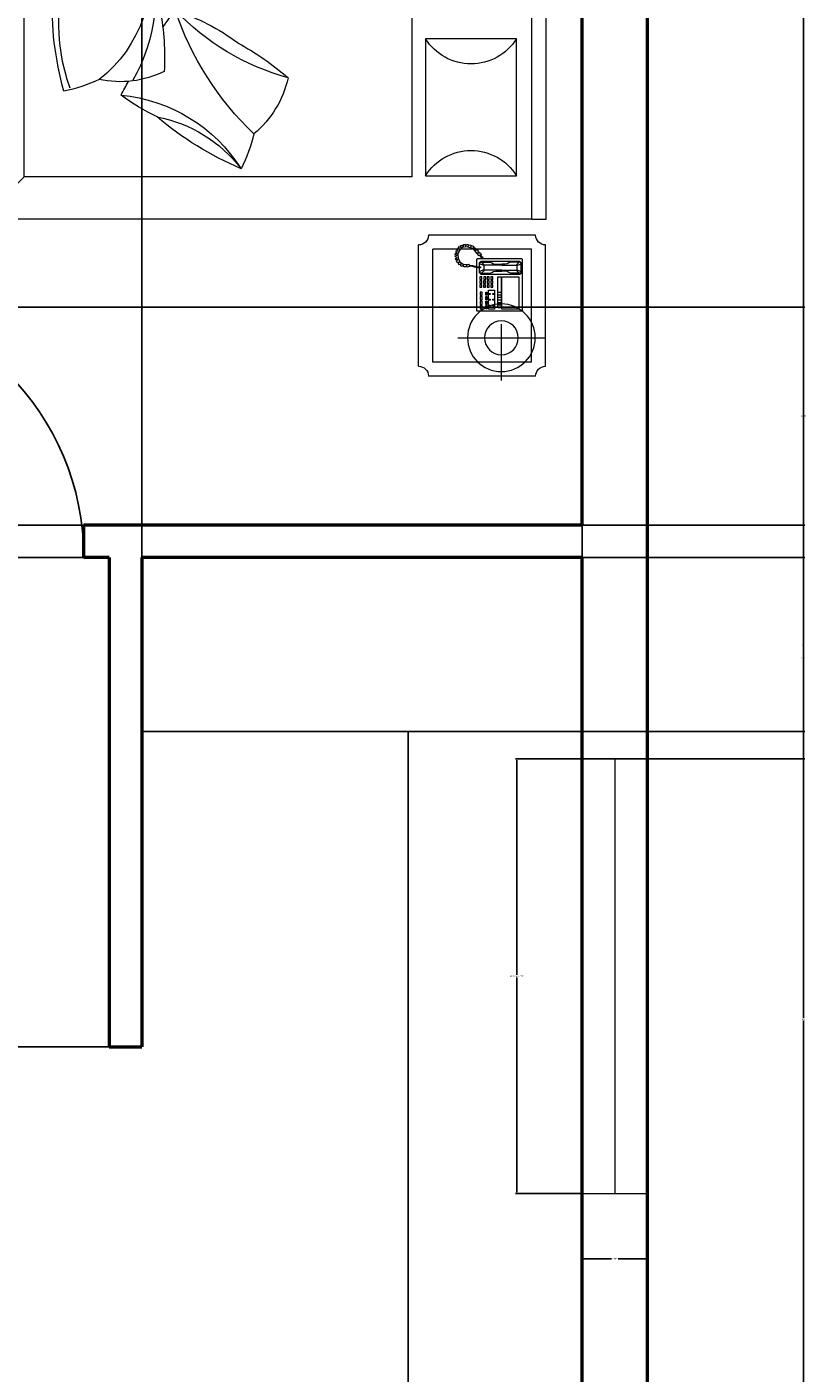
# Model space of a CAD drawing. Units: inches. Extents: x -108 to 1456, y -102 to 617.
# Tile 6 of 8: x 453 to 560, y 337 to 523. Entities that reach past the tile are written whole.
import ezdxf

# ---------------------------------------------------------------- set-up
doc = ezdxf.new("R2010")
doc.units = ezdxf.units.IN
for name, color, linetype, lineweight in [('A-ANNO-DIMS', 2, 'Continuous', 18), ('A-DOOR', 3, 'Continuous', 25), ('A-FLOR-CASE', 32, 'Continuous', 25), ('A-FURN', 8, 'Continuous', 18), ('A-GLAZ', 4, 'Continuous', 18), ('A-WALL', 7, 'Continuous', 50)]:
    doc.layers.add(name, color=color, linetype=linetype, lineweight=lineweight)
doc.styles.get("Standard").update_dxf_attribs({"font": 'arial.ttf'})
doc.dimstyles.get("Standard").update_dxf_attribs({"dimtxt": 0.18, "dimasz": 0.18, "dimexe": 0.18, "dimexo": 0.0625, "dimgap": 0.09, "dimtad": 0, "dimtih": 1, "dimtoh": 1, "dimdec": 4, "dimzin": 0, "dimdsep": 46, "dimtxsty": 'Standard', "dimcen": 0.09, "dimadec": 0, "dimazin": 0, "dimtfac": 1, "dimtdec": 4, "dimtofl": 0, "dimtmove": 0, "dimatfit": 3, "dimfxl": 1, "dimtolj": 1, "dimtzin": 0, "dimarcsym": 0})

# ---------------------------------------------------------------- blocks, each defined once
blk = doc.blocks.new('A$C50B66110')
for p, q in [((0.0153, 1.9631), (0.0153, 1.5831)), ((0.0503, 1.9981), (0.4803, 1.9981)), ((0.1513, 1.6871), (0.1513, 1.9967)), ((0.5153, 1.9631), (0.5153, 1.5831)), ((0.5716, 1.9488), (0.5716, 2)), ((0.5716, 2), (2.0719, 2)), ((2.0719, 1.9488), (2.0719, 2)), ((2.1051, 1.9643), (2.1051, 1.5843)), ((2.5701, 1.9993), (2.1401, 1.9993)), ((2.6051, 1.9643), (2.6051, 1.5843)), ((0.0653, 1.9481), (0.0653, 1.5981)), ((0.0653, 1.9481), (0.4653, 1.9481)), ((0.4653, 1.9481), (0.4653, 1.5981)), ((2.0719, 1.9488), (0.5716, 1.9488)), ((0.5716, 1.9488), (0.5716, 0)), ((2.0719, 0), (2.0719, 1.9488)), ((2.1551, 1.9493), (2.1551, 1.5993)), ((2.5551, 1.9493), (2.1551, 1.9493)), ((2.3505, 1.62), (2.3505, 1.9295)), ((2.5551, 1.9493), (2.5551, 1.5993)), ((0.7257, 1.5725), (0.7257, 1.8954)), ((0.7257, 1.8954), (1.2113, 1.8954)), ((1.2113, 1.8954), (1.2113, 1.5725)), ((1.4007, 1.5725), (1.4007, 1.8954)), ((1.4007, 1.8954), (1.8863, 1.8954)), ((1.8863, 1.8954), (1.8863, 1.5725)), ((0, 1.8416), (0.2001, 1.8416)), ((2.5018, 1.7744), (2.2017, 1.7744)), ((0.0653, 1.5981), (0.4653, 1.5981)), ((2.5551, 1.5993), (2.1551, 1.5993)), ((0.0503, 1.5481), (0.4803, 1.5481)), ((1.2113, 1.5725), (0.7257, 1.5725)), ((1.8863, 1.5725), (1.4007, 1.5725)), ((2.5701, 1.5493), (2.1401, 1.5493)), ((1.5665, 1.5254), (1.5665, 1.0802)), ((1.5665, 1.5254), (1.9219, 1.0802)), ((1.9219, 1.0802), (1.5665, 1.0802)), ((0.5716, 0), (0.7216, 0.15)), ((2.0719, 0), (1.9219, 0.15)), ((0.5716, 0), (2.0719, 0))]:
    blk.add_line(p, q)
at = {"linetype": 'ByBlock'}
for p, q in [((0.2481, 1.9162), (0.2458, 1.9139)), ((0.2458, 1.9139), (0.2458, 1.7562)), ((0.2481, 1.9162), (0.4287, 1.9162)), ((0.3772, 1.9071), (0.3818, 1.9128)), ((0.3818, 1.9094), (0.3807, 1.9048)), ((0.3818, 1.9128), (0.4161, 1.9128)), ((0.3864, 1.9116), (0.3818, 1.9094)), ((0.3921, 1.8968), (0.3864, 1.9116)), ((0.3864, 1.9116), (0.4138, 1.9116)), ((0.4081, 1.8968), (0.4138, 1.9116)), ((0.4138, 1.9116), (0.4184, 1.9094)), ((0.4161, 1.9128), (0.4218, 1.9071)), ((0.4184, 1.9094), (0.4195, 1.9048)), ((0.4287, 1.9162), (0.4309, 1.9139)), ((0.4309, 1.9139), (0.4309, 1.7562)), ((0.2526, 1.9036), (0.2526, 1.8431)), ((0.3669, 1.9036), (0.2526, 1.9036)), ((0.3669, 1.8431), (0.3669, 1.9036)), ((0.3772, 1.7688), (0.3772, 1.9071)), ((0.3807, 1.9048), (0.3807, 1.8739)), ((0.3807, 1.9048), (0.3909, 1.8945)), ((0.3807, 1.8739), (0.3829, 1.8682)), ((0.3829, 1.8682), (0.3864, 1.8625)), ((0.3864, 1.8625), (0.3875, 1.8545)), ((0.3909, 1.8945), (0.3921, 1.8968)), ((0.3909, 1.8431), (0.3909, 1.8945)), ((0.4081, 1.8968), (0.3921, 1.8968)), ((0.4092, 1.8945), (0.4081, 1.8968)), ((0.4195, 1.9048), (0.4092, 1.8945)), ((0.4092, 1.8431), (0.4092, 1.8945)), ((0.4138, 1.8625), (0.4127, 1.8545)), ((0.4172, 1.8682), (0.4138, 1.8625)), ((0.4195, 1.8739), (0.4172, 1.8682)), ((0.4195, 1.9048), (0.4195, 1.8739)), ((0.4218, 1.9071), (0.4218, 1.7699)), ((0.2526, 1.8431), (0.3669, 1.8431)), ((0.3201, 1.8168), (0.2526, 1.8168)), ((0.2526, 1.8168), (0.2526, 1.7962)), ((0.2572, 1.8408), (0.2572, 1.8294)), ((0.3669, 1.8408), (0.2572, 1.8408)), ((0.2572, 1.8294), (0.3669, 1.8294)), ((0.2675, 1.8145), (0.2641, 1.8145)), ((0.2641, 1.8145), (0.2641, 1.8111)), ((0.2664, 1.8408), (0.2664, 1.8294)), ((0.2675, 1.8111), (0.2675, 1.8145)), ((0.2755, 1.8408), (0.2755, 1.8294)), ((0.2846, 1.8408), (0.2846, 1.8294)), ((0.2846, 1.8145), (0.2846, 1.8111)), ((0.2881, 1.8145), (0.2846, 1.8145)), ((0.2881, 1.8111), (0.2881, 1.8145)), ((0.2938, 1.8408), (0.2938, 1.8294)), ((0.3029, 1.8408), (0.3029, 1.8294)), ((0.3052, 1.8145), (0.3052, 1.8111)), ((0.3086, 1.8145), (0.3052, 1.8145)), ((0.3086, 1.8111), (0.3086, 1.8145)), ((0.3121, 1.8408), (0.3121, 1.8294)), ((0.3201, 1.7962), (0.3201, 1.8168)), ((0.3669, 1.8294), (0.3669, 1.8408)), ((0.3829, 1.8076), (0.3864, 1.8134)), ((0.3864, 1.8134), (0.3875, 1.8214)), ((0.3875, 1.8545), (0.3875, 1.8431)), ((0.3875, 1.8214), (0.3875, 1.8431)), ((0.3909, 1.8431), (0.3909, 1.7813)), ((0.4092, 1.8431), (0.4092, 1.7813)), ((0.4127, 1.8545), (0.4127, 1.8431)), ((0.4127, 1.8214), (0.4127, 1.8431)), ((0.4138, 1.8134), (0.4127, 1.8214)), ((0.4172, 1.8076), (0.4138, 1.8134)), ((0.2526, 1.7962), (0.3201, 1.7962)), ((0.2652, 1.7905), (0.2538, 1.7905)), ((0.2538, 1.7905), (0.2538, 1.7859)), ((0.2538, 1.7859), (0.2652, 1.7859)), ((0.2538, 1.7665), (0.2538, 1.7733)), ((0.2538, 1.7733), (0.2652, 1.7733)), ((0.2652, 1.7665), (0.2538, 1.7665)), ((0.2641, 1.8111), (0.2675, 1.8111)), ((0.2641, 1.8019), (0.2641, 1.7985)), ((0.2675, 1.8019), (0.2641, 1.8019)), ((0.2641, 1.7985), (0.2675, 1.7985)), ((0.2652, 1.7859), (0.2652, 1.7905)), ((0.2652, 1.7733), (0.2652, 1.7665)), ((0.2675, 1.7985), (0.2675, 1.8019)), ((0.2812, 1.7905), (0.2698, 1.7905)), ((0.2698, 1.7905), (0.2698, 1.7859)), ((0.2698, 1.7859), (0.2812, 1.7859)), ((0.2698, 1.7665), (0.2698, 1.7733)), ((0.2698, 1.7733), (0.2812, 1.7733)), ((0.2812, 1.7665), (0.2698, 1.7665)), ((0.2812, 1.7859), (0.2812, 1.7905)), ((0.2812, 1.7733), (0.2812, 1.7665)), ((0.2846, 1.8111), (0.2881, 1.8111)), ((0.2846, 1.8019), (0.2846, 1.7985)), ((0.2881, 1.8019), (0.2846, 1.8019)), ((0.2846, 1.7985), (0.2881, 1.7985)), ((0.2972, 1.7905), (0.2858, 1.7905)), ((0.2858, 1.7905), (0.2858, 1.7859)), ((0.2858, 1.7859), (0.2972, 1.7859)), ((0.2858, 1.7665), (0.2858, 1.7733)), ((0.2858, 1.7733), (0.2972, 1.7733)), ((0.2972, 1.7665), (0.2858, 1.7665)), ((0.2881, 1.7985), (0.2881, 1.8019)), ((0.2972, 1.7859), (0.2972, 1.7905)), ((0.2972, 1.7733), (0.2972, 1.7665)), ((0.3018, 1.7905), (0.3018, 1.7859)), ((0.3132, 1.7905), (0.3018, 1.7905)), ((0.3018, 1.7859), (0.3132, 1.7859)), ((0.3018, 1.7733), (0.3132, 1.7733)), ((0.3018, 1.7665), (0.3018, 1.7733)), ((0.3132, 1.7665), (0.3018, 1.7665)), ((0.3052, 1.8111), (0.3086, 1.8111)), ((0.3052, 1.8019), (0.3052, 1.7985)), ((0.3086, 1.8019), (0.3052, 1.8019)), ((0.3052, 1.7985), (0.3086, 1.7985)), ((0.3086, 1.7985), (0.3086, 1.8019)), ((0.3132, 1.7859), (0.3132, 1.7905)), ((0.3132, 1.7733), (0.3132, 1.7665)), ((0.3304, 1.8111), (0.3395, 1.8111)), ((0.3304, 1.8042), (0.3304, 1.8111)), ((0.3395, 1.8042), (0.3304, 1.8042)), ((0.3304, 1.7985), (0.3395, 1.7985)), ((0.3304, 1.7916), (0.3304, 1.7985)), ((0.3395, 1.7916), (0.3304, 1.7916)), ((0.3304, 1.7779), (0.3304, 1.7848)), ((0.3304, 1.7848), (0.3395, 1.7848)), ((0.3395, 1.7779), (0.3304, 1.7779)), ((0.3304, 1.7722), (0.3395, 1.7722)), ((0.3304, 1.7653), (0.3304, 1.7722)), ((0.3395, 1.8111), (0.3395, 1.8042)), ((0.3395, 1.7985), (0.3395, 1.7916)), ((0.3395, 1.7848), (0.3395, 1.7779)), ((0.3395, 1.7722), (0.3395, 1.7653)), ((0.3441, 1.8042), (0.3441, 1.8111)), ((0.3441, 1.8111), (0.3532, 1.8111)), ((0.3532, 1.8042), (0.3441, 1.8042)), ((0.3441, 1.7985), (0.3532, 1.7985)), ((0.3441, 1.7916), (0.3441, 1.7985)), ((0.3532, 1.7916), (0.3441, 1.7916)), ((0.3441, 1.7779), (0.3441, 1.7848)), ((0.3441, 1.7848), (0.3532, 1.7848)), ((0.3532, 1.7779), (0.3441, 1.7779)), ((0.3441, 1.7722), (0.3532, 1.7722)), ((0.3441, 1.7653), (0.3441, 1.7722)), ((0.3532, 1.8111), (0.3532, 1.8042)), ((0.3532, 1.7985), (0.3532, 1.7916)), ((0.3532, 1.7848), (0.3532, 1.7779)), ((0.3532, 1.7722), (0.3532, 1.7653)), ((0.3578, 1.8111), (0.3669, 1.8111)), ((0.3578, 1.8042), (0.3578, 1.8111)), ((0.3669, 1.8042), (0.3578, 1.8042)), ((0.3578, 1.7985), (0.3669, 1.7985)), ((0.3578, 1.7916), (0.3578, 1.7985)), ((0.3669, 1.7916), (0.3578, 1.7916)), ((0.3578, 1.7791), (0.3578, 1.7859)), ((0.3578, 1.7859), (0.3669, 1.7859)), ((0.3669, 1.7791), (0.3578, 1.7791)), ((0.3578, 1.7653), (0.3578, 1.7722)), ((0.3578, 1.7722), (0.3669, 1.7722)), ((0.3669, 1.8111), (0.3669, 1.8042)), ((0.3669, 1.7985), (0.3669, 1.7916)), ((0.3669, 1.7859), (0.3669, 1.7791)), ((0.3669, 1.7722), (0.3669, 1.7653)), ((0.3829, 1.7631), (0.3772, 1.7688)), ((0.3807, 1.8019), (0.3829, 1.8076)), ((0.3807, 1.7711), (0.3807, 1.8019)), ((0.3807, 1.7711), (0.3909, 1.7813)), ((0.3818, 1.7665), (0.3807, 1.7711)), ((0.3864, 1.7642), (0.3818, 1.7665)), ((0.3921, 1.7791), (0.3864, 1.7642)), ((0.3909, 1.7813), (0.3921, 1.7791)), ((0.4081, 1.7791), (0.3921, 1.7791)), ((0.4024, 1.7676), (0.3989, 1.7676)), ((0.3989, 1.7676), (0.3991, 1.7578)), ((0.403, 1.7585), (0.4024, 1.7676)), ((0.4092, 1.7813), (0.4081, 1.7791)), ((0.4081, 1.7791), (0.4138, 1.7642)), ((0.4195, 1.7711), (0.4092, 1.7813)), ((0.4138, 1.7642), (0.4184, 1.7665)), ((0.4218, 1.7699), (0.4161, 1.7631)), ((0.4195, 1.8019), (0.4172, 1.8076)), ((0.4184, 1.7665), (0.4195, 1.7711)), ((0.4195, 1.7711), (0.4195, 1.8019)), ((0.4378, 1.7742), (0.4309, 1.7768)), ((0.4309, 1.7722), (0.436, 1.7708)), ((0.436, 1.7708), (0.4406, 1.7672)), ((0.441, 1.771), (0.4378, 1.7742)), ((0.4406, 1.7672), (0.4418, 1.7656)), ((0.4434, 1.7688), (0.441, 1.771)), ((0.4443, 1.7658), (0.4418, 1.7633)), ((0.4418, 1.7656), (0.4443, 1.7658)), ((0.4477, 1.7704), (0.4434, 1.7688)), ((0.4497, 1.7684), (0.4477, 1.7704)), ((0.4481, 1.765), (0.4497, 1.7684)), ((0.4509, 1.7672), (0.4481, 1.765)), ((0.4539, 1.764), (0.4509, 1.7672)), ((0.2458, 1.7562), (0.2481, 1.7539)), ((0.4, 1.7539), (0.2481, 1.7539)), ((0.3395, 1.7653), (0.3304, 1.7653)), ((0.3532, 1.7653), (0.3441, 1.7653)), ((0.3669, 1.7653), (0.3578, 1.7653)), ((0.399, 1.7631), (0.3829, 1.7631)), ((0.3864, 1.7642), (0.399, 1.7642)), ((0.3991, 1.7578), (0.4019, 1.7462)), ((0.4019, 1.7462), (0.4047, 1.7353)), ((0.4026, 1.7254), (0.4021, 1.7198)), ((0.4021, 1.7198), (0.4088, 1.7187)), ((0.4088, 1.7187), (0.4023, 1.7147)), ((0.4026, 1.7642), (0.4138, 1.7642)), ((0.4051, 1.7279), (0.4026, 1.7254)), ((0.4161, 1.7631), (0.4027, 1.7631)), ((0.4047, 1.7511), (0.403, 1.7585)), ((0.4287, 1.7539), (0.404, 1.7539)), ((0.4047, 1.7353), (0.4044, 1.7293)), ((0.4044, 1.7293), (0.4051, 1.7279)), ((0.4074, 1.7402), (0.4047, 1.7511)), ((0.4081, 1.7346), (0.4074, 1.7402)), ((0.4079, 1.7286), (0.4081, 1.7346)), ((0.4121, 1.7256), (0.4079, 1.7286)), ((0.4111, 1.7203), (0.4121, 1.7256)), ((0.4123, 1.7057), (0.4111, 1.7203)), ((0.4309, 1.7562), (0.4287, 1.7539)), ((0.4418, 1.7633), (0.4511, 1.7551)), ((0.4511, 1.7551), (0.4662, 1.7422)), ((0.4515, 1.7573), (0.4539, 1.764)), ((0.4577, 1.7605), (0.4515, 1.7573)), ((0.463, 1.7555), (0.4577, 1.7605)), ((0.4618, 1.7482), (0.463, 1.7555)), ((0.467, 1.7515), (0.4618, 1.7482)), ((0.4664, 1.7418), (0.4741, 1.72)), ((0.4714, 1.7468), (0.467, 1.7515)), ((0.4696, 1.7418), (0.4714, 1.7468)), ((0.4766, 1.7425), (0.4697, 1.7418)), ((0.4741, 1.72), (0.4708, 1.7027)), ((0.472, 1.733), (0.4787, 1.7356)), ((0.4794, 1.7332), (0.472, 1.733)), ((0.4761, 1.7233), (0.481, 1.7279)), ((0.4824, 1.7233), (0.4761, 1.7233)), ((0.4787, 1.7356), (0.4766, 1.7425)), ((0.481, 1.7279), (0.4794, 1.7332)), ((0.4835, 1.7175), (0.4824, 1.7233)), ((0.4023, 1.7147), (0.4028, 1.7085)), ((0.4028, 1.7085), (0.4102, 1.7078)), ((0.4102, 1.7078), (0.4037, 1.7027)), ((0.4037, 1.7027), (0.4067, 1.6974)), ((0.4067, 1.6974), (0.4137, 1.6988)), ((0.4137, 1.6988), (0.4104, 1.6923)), ((0.4104, 1.6923), (0.4139, 1.6881)), ((0.4211, 1.6946), (0.4123, 1.7057)), ((0.4139, 1.6881), (0.4192, 1.692)), ((0.4192, 1.692), (0.4183, 1.6858)), ((0.4183, 1.6858), (0.4227, 1.683)), ((0.4333, 1.6881), (0.4211, 1.6946)), ((0.4227, 1.683), (0.4283, 1.6876)), ((0.4283, 1.6876), (0.4276, 1.68)), ((0.4276, 1.68), (0.4324, 1.6786)), ((0.4324, 1.6786), (0.4354, 1.6849)), ((0.4472, 1.6869), (0.4333, 1.6881)), ((0.4354, 1.6849), (0.4382, 1.6786)), ((0.4382, 1.6786), (0.4421, 1.6782)), ((0.4421, 1.6782), (0.4437, 1.6849)), ((0.4437, 1.6849), (0.4463, 1.6775)), ((0.4463, 1.6775), (0.4507, 1.6786)), ((0.4606, 1.6927), (0.4472, 1.6869)), ((0.4507, 1.6786), (0.4509, 1.6849)), ((0.4509, 1.6849), (0.4562, 1.6802)), ((0.4562, 1.6802), (0.4599, 1.6821)), ((0.4592, 1.689), (0.4641, 1.683)), ((0.4599, 1.6821), (0.4592, 1.689)), ((0.4708, 1.7027), (0.4606, 1.6927)), ((0.4641, 1.683), (0.4678, 1.6863)), ((0.465, 1.6925), (0.4715, 1.6897)), ((0.4678, 1.6863), (0.465, 1.6925)), ((0.4745, 1.6925), (0.4713, 1.6988)), ((0.4713, 1.6988), (0.478, 1.6967)), ((0.4715, 1.6897), (0.4745, 1.6925)), ((0.4743, 1.7075), (0.4815, 1.7073)), ((0.4798, 1.7013), (0.4743, 1.7075)), ((0.4764, 1.7154), (0.4835, 1.7175)), ((0.4824, 1.7119), (0.4764, 1.7154)), ((0.478, 1.6967), (0.4798, 1.7013)), ((0.4815, 1.7073), (0.4824, 1.7119)), ((0.7216, 1.5254), (1.9219, 1.5254)), ((0.7216, 1.5254), (0.7216, 0.15)), ((1.9219, 0.15), (1.9219, 1.5254)), ((0.7216, 0.15), (1.9219, 0.15))]:
    blk.add_line(p, q, dxfattribs=at)
for centre, radius in [((0.1513, 1.8416), 0.12), ((0.1513, 1.8416), 0.06), ((2.3505, 1.7744), 0.12), ((2.3505, 1.7744), 0.06)]:
    blk.add_circle(centre, radius)
for centre, radius, start, end in [((0.0153, 1.9981), 0.035, 270, 0), ((0.5153, 1.9981), 0.035, 180, 270), ((2.1051, 1.9993), 0.035, 270, 0), ((2.6051, 1.9993), 0.035, 180, 270), ((0.6244, 1.734), 0.1906, 302.1202, 57.8798), ((1.3126, 1.734), 0.1906, 122.1202, 237.8798), ((1.2994, 1.734), 0.1906, 302.1202, 57.8798), ((1.9876, 1.734), 0.1906, 122.1202, 237.8798), ((0.0153, 1.5481), 0.035, 0, 90), ((0.5153, 1.5481), 0.035, 90, 180), ((2.1051, 1.5493), 0.035, 0, 90), ((2.6051, 1.5493), 0.035, 90, 180), ((1.1502, 0.7366), 0.3575, 102.4782, 140.4625), ((0.328, 0.4368), 0.9879, 28.4971, 41.0566), ((1.9117, 1.3157), 0.8697, 195.336, 226.4193), ((0.9996, 0.4307), 0.548, 103.2034, 117.0362), ((1.656, 1.7093), 1.0798, 223.6306, 251.4288), ((0.4482, 0.4408), 0.5655, 5.3391, 57.6895), ((1.8226, 1.3753), 1.1652, 203.0642, 220.3209), ((0.4548, 0.5307), 0.4879, 10.6986, 52.6864), ((0.5648, 0.4378), 0.7874, 18.3527, 36.6851), ((-0.0179, 2.4352), 2.1977, 305.2966, 307.2418), ((1.5981, 0.9345), 0.734, 205.259, 216.9351), ((1.4166, 0.4903), 0.3575, 154.0418, 192.0262), ((1.1403, -0.3401), 0.9879, 80.0607, 92.6202), ((1.2867, -0.154), 0.7874, 69.9163, 88.2487), ((1.3672, 0.0075), 0.6085, 71.81, 120.1351), ((1.4431, 0.1219), 0.4774, 76.1849, 142.0017), ((-0.6401, 0.6314), 2.1977, 349.4884, 358.8054), ((-0.0179, 2.4352), 2.1977, 297.9248, 299.3793), ((1.5626, 0.1822), 0.548, 154.767, 168.5998), ((1.3343, 1.4141), 1.1652, 254.6278, 271.8845), ((1.2678, 0.9611), 0.6885, 250.2936, 293.6414), ((1.5399, 0.9642), 0.734, 256.8226, 268.4988)]:
    blk.add_arc(centre, radius, start, end)
blk = doc.blocks.new('WIN-60-WALL-9')
for p, q in [((0, 0), (0, 9)), ((60, 0), (60, 9)), ((0, 4.5), (60, 4.5))]:
    blk.add_line(p, q)
blk = doc.blocks.new('*D16')
at = {"layer": 'A-ANNO-DIMS', "color": 0, "lineweight": -2, "transparency": 16777216}
for p, q in [((529.28, 421.77), (520.16, 421.77)), ((520.34, 421.59), (520.34, 391.96)), ((520.34, 361.95), (520.34, 391.59)), ((529.28, 361.77), (520.16, 361.77))]:
    blk.add_line(p, q, dxfattribs=at)
at = {"layer": 'A-ANNO-DIMS', "color": 0, "transparency": 16777216}
for points in [[(520.31, 421.59), (520.37, 421.59), (520.34, 421.77)], [(520.31, 361.95), (520.37, 361.95), (520.34, 361.77)]]:
    blk.add_solid(points, dxfattribs=at)
at = {"layer": 'Defpoints', "color": 0, "transparency": 16777216}
for p in [(529.34, 421.77), (520.34, 361.77), (529.34, 361.77)]:
    blk.add_point(p, dxfattribs=at)
at = {"layer": 'A-ANNO-DIMS', "color": 0, "transparency": 16777216, "insert": (520.34, 391.77), "char_height": 0.18, "attachment_point": 5}
blk.add_mtext('\\A1;WINDOW 60 TYP.', dxfattribs=at)
blk = doc.blocks.new('*D17')
at = {"layer": 'A-ANNO-DIMS', "color": 0, "lineweight": -2, "transparency": 16777216}
for p, q in [((529.34, 361.71), (529.34, 352.59)), ((538.34, 361.71), (538.34, 352.59)), ((529.52, 352.77), (533.39, 352.77)), ((538.16, 352.77), (534.3, 352.77))]:
    blk.add_line(p, q, dxfattribs=at)
at = {"layer": 'A-ANNO-DIMS', "color": 0, "transparency": 16777216}
for points in [[(529.52, 352.8), (529.52, 352.74), (529.34, 352.77)], [(538.16, 352.8), (538.16, 352.74), (538.34, 352.77)]]:
    blk.add_solid(points, dxfattribs=at)
at = {"layer": 'Defpoints', "color": 0, "transparency": 16777216}
for p in [(529.34, 361.77), (538.34, 361.77), (538.34, 352.77)]:
    blk.add_point(p, dxfattribs=at)
at = {"layer": 'A-ANNO-DIMS', "color": 0, "transparency": 16777216, "insert": (533.84, 352.77), "char_height": 0.18, "attachment_point": 5}
blk.add_mtext('\\A1;9 TYP.', dxfattribs=at)
blk = doc.blocks.new('*D35')
at = {"layer": 'A-ANNO-DIMS', "color": 0, "lineweight": -2, "transparency": 16777216}
for p, q in [((538.41, 595.77), (560.05, 595.77)), ((559.87, 595.59), (559.87, 385.96)), ((559.87, 175.95), (559.87, 385.59)), ((538.41, 175.77), (560.05, 175.77))]:
    blk.add_line(p, q, dxfattribs=at)
at = {"layer": 'A-ANNO-DIMS', "color": 0, "transparency": 16777216}
for points in [[(559.84, 595.59), (559.9, 595.59), (559.87, 595.77)], [(559.84, 175.95), (559.9, 175.95), (559.87, 175.77)]]:
    blk.add_solid(points, dxfattribs=at)
at = {"layer": 'Defpoints', "color": 0, "transparency": 16777216}
for p in [(538.34, 595.77), (559.87, 595.77), (538.34, 175.77)]:
    blk.add_point(p, dxfattribs=at)
at = {"layer": 'A-ANNO-DIMS', "color": 0, "transparency": 16777216, "insert": (559.87, 385.77), "char_height": 0.18, "attachment_point": 5}
blk.add_mtext('\\A1;420', dxfattribs=at)
blk = doc.blocks.new('*D52')
at = {"layer": 'A-ANNO-DIMS', "color": 0, "lineweight": -2, "transparency": 16777216}
for p, q in [((415.48, 484.07), (560.05, 484.07)), ((559.87, 483.89), (559.87, 469.23)), ((559.87, 454.2), (559.87, 468.86)), ((416.16, 454.02), (560.05, 454.02))]:
    blk.add_line(p, q, dxfattribs=at)
at = {"layer": 'A-ANNO-DIMS', "color": 0, "transparency": 16777216}
for points in [[(559.84, 483.89), (559.9, 483.89), (559.87, 484.07)], [(559.84, 454.2), (559.9, 454.2), (559.87, 454.02)]]:
    blk.add_solid(points, dxfattribs=at)
at = {"layer": 'Defpoints', "color": 0, "transparency": 16777216}
for p in [(415.41, 484.07), (416.09, 454.02), (559.87, 454.02)]:
    blk.add_point(p, dxfattribs=at)
at = {"layer": 'A-ANNO-DIMS', "color": 0, "transparency": 16777216, "insert": (559.87, 469.05), "char_height": 0.18, "attachment_point": 5}
blk.add_mtext('\\A1;30.044', dxfattribs=at)
blk = doc.blocks.new('*D54')
at = {"layer": 'A-ANNO-DIMS', "color": 0, "lineweight": -2, "transparency": 16777216}
for p, q in [((529.41, 449.52), (560.05, 449.52)), ((559.87, 449.34), (559.87, 435.83)), ((559.87, 421.95), (559.87, 435.47)), ((529.41, 421.77), (560.05, 421.77))]:
    blk.add_line(p, q, dxfattribs=at)
at = {"layer": 'A-ANNO-DIMS', "color": 0, "transparency": 16777216}
for points in [[(559.84, 449.34), (559.9, 449.34), (559.87, 449.52)], [(559.84, 421.95), (559.9, 421.95), (559.87, 421.77)]]:
    blk.add_solid(points, dxfattribs=at)
at = {"layer": 'Defpoints', "color": 0, "transparency": 16777216}
for p in [(529.34, 449.52), (529.34, 421.77), (559.87, 421.77)]:
    blk.add_point(p, dxfattribs=at)
at = {"layer": 'A-ANNO-DIMS', "color": 0, "transparency": 16777216, "insert": (559.87, 435.65), "char_height": 0.18, "attachment_point": 5}
blk.add_mtext('\\A1;27.75', dxfattribs=at)
blk = doc.blocks.new('*D57')
at = {"layer": 'A-ANNO-DIMS', "color": 0, "lineweight": -2, "transparency": 16777216}
for p, q in [((468.59, 449.59), (468.59, 617.48)), ((468.77, 617.3), (498.57, 617.3)), ((529.16, 617.3), (499.36, 617.3)), ((529.34, 449.59), (529.34, 617.48))]:
    blk.add_line(p, q, dxfattribs=at)
at = {"layer": 'A-ANNO-DIMS', "color": 0, "transparency": 16777216}
for points in [[(468.77, 617.33), (468.77, 617.27), (468.59, 617.3)], [(529.16, 617.33), (529.16, 617.27), (529.34, 617.3)]]:
    blk.add_solid(points, dxfattribs=at)
at = {"layer": 'Defpoints', "color": 0, "transparency": 16777216}
for p in [(529.34, 617.3), (468.59, 449.52), (529.34, 449.52)]:
    blk.add_point(p, dxfattribs=at)
at = {"layer": 'A-ANNO-DIMS', "color": 0, "transparency": 16777216, "insert": (498.97, 617.3), "char_height": 0.18, "attachment_point": 5}
blk.add_mtext('\\A1;60.75', dxfattribs=at)
blk = doc.blocks.new('*D58')
at = {"layer": 'A-ANNO-DIMS', "color": 0, "lineweight": -2, "transparency": 16777216}
for p, q in [((464.03, 449.52), (204.64, 449.52)), ((204.82, 449.34), (204.82, 415.95)), ((204.82, 382.19), (204.82, 415.58)), ((464.03, 382.01), (204.64, 382.01))]:
    blk.add_line(p, q, dxfattribs=at)
at = {"layer": 'A-ANNO-DIMS', "color": 0, "transparency": 16777216}
for points in [[(204.79, 449.34), (204.85, 449.34), (204.82, 449.52)], [(204.79, 382.19), (204.85, 382.19), (204.82, 382.01)]]:
    blk.add_solid(points, dxfattribs=at)
at = {"layer": 'Defpoints', "color": 0, "transparency": 16777216}
for p in [(464.09, 449.52), (204.82, 382.01), (464.09, 382.01)]:
    blk.add_point(p, dxfattribs=at)
at = {"layer": 'A-ANNO-DIMS', "color": 0, "transparency": 16777216, "insert": (204.82, 415.77), "char_height": 0.18, "attachment_point": 5}
blk.add_mtext('\\A1;67.52', dxfattribs=at)
blk = doc.blocks.new('*D60')
at = {"layer": 'A-ANNO-DIMS', "color": 0, "lineweight": -2, "transparency": 16777216}
for p, q in [((468.66, 449.52), (560.05, 449.52)), ((559.87, 449.34), (559.87, 437.7)), ((559.87, 425.7), (559.87, 437.34)), ((468.66, 425.52), (560.05, 425.52))]:
    blk.add_line(p, q, dxfattribs=at)
at = {"layer": 'A-ANNO-DIMS', "color": 0, "transparency": 16777216}
for points in [[(559.84, 449.34), (559.9, 449.34), (559.87, 449.52)], [(559.84, 425.7), (559.9, 425.7), (559.87, 425.52)]]:
    blk.add_solid(points, dxfattribs=at)
at = {"layer": 'Defpoints', "color": 0, "transparency": 16777216}
for p in [(468.59, 449.52), (559.87, 449.52), (468.59, 425.52)]:
    blk.add_point(p, dxfattribs=at)
at = {"layer": 'A-ANNO-DIMS', "color": 0, "transparency": 16777216, "insert": (559.87, 437.52), "char_height": 0.18, "attachment_point": 5}
blk.add_mtext('\\A1;24', dxfattribs=at)

msp = doc.modelspace()

# ---------------------------------------------------------------- linework, layer by layer
at = {"layer": 'A-DOOR'}
msp.add_arc((424.5943, 449.5243), 36, 0, 90, dxfattribs=at)
at = {"layer": 'A-FLOR-CASE'}
for p, q in [((468.5943, 449.5243), (529.3443, 449.5243)), ((529.3443, 449.5243), (511.794, 449.5243)), ((468.5943, 425.5243), (529.3443, 425.5243)), ((505.3443, 334.021), (505.3443, 425.5243)), ((529.3443, 334.021), (529.3443, 425.5243))]:
    msp.add_line(p, q, dxfattribs=at)
at = {"layer": 'A-WALL'}
for p, q in [((538.3443, 175.7743), (538.3443, 595.7743)), ((529.3443, 454.0243), (529.3443, 586.7743)), ((529.3443, 454.0243), (460.5943, 454.0243)), ((460.5943, 449.5243), (460.5943, 454.0243)), ((464.0943, 449.5243), (460.5943, 449.5243)), ((464.0943, 449.5243), (464.0943, 382.0065)), ((529.3443, 449.5243), (468.5943, 449.5243)), ((468.5943, 449.5243), (468.5943, 382.0076)), ((529.3443, 334.021), (529.3443, 449.5243)), ((464.0943, 382.0065), (468.5943, 382.0076))]:
    msp.add_line(p, q, dxfattribs=at)

# ---------------------------------------------------------------- block references
at = {"layer": 'A-FURN', "xscale": -38.92841910804861, "yscale": 38.92841910804861, "zscale": 38.92841910804861, "rotation": 270}
msp.add_blockref('A$C50B66110', (446.5101, 473.9691), dxfattribs=at)
at = {"layer": 'A-GLAZ', "rotation": 270}
msp.add_blockref('WIN-60-WALL-9', (529.344, 421.7746), dxfattribs=at)

# ---------------------------------------------------------------- dimensions: what is measured, and where the dimension line sits
at = {"layer": 'A-ANNO-DIMS'}
dim = msp.add_linear_dim(base=(529.3443, 617.2993), p1=(468.5943, 449.5243), p2=(529.3443, 449.5243), dimstyle='Standard', override={"dimdec": 2, "dimlfac": 1, "dimrnd": 0, "dimzin": 0, "dimdsep": 46, "dimlunit": 2}, dxfattribs=at)
dim.commit()
dim.dimension.update_dxf_attribs({"geometry": '*D57', "text_midpoint": (498.9693, 617.2993)})
for base, p1, p2, override, picture, middle in [((559.8693, 595.7743), (538.3443, 175.7743), (538.3443, 595.7743), {"dimdec": 0, "dimlfac": 1, "dimrnd": 0, "dimzin": 0, "dimdsep": 46, "dimlunit": 2}, '*D35', (559.8693, 385.7743)), ((559.8693, 454.0243), (415.4127, 484.0682), (416.0943, 454.0243), {"dimdec": 3, "dimlfac": 1, "dimrnd": 0, "dimzin": 0, "dimdsep": 46, "dimlunit": 2}, '*D52', (559.8693, 469.0462)), ((204.8193, 382.0065), (464.0943, 449.5243), (464.0943, 382.0065), {"dimdec": 2, "dimlfac": 1, "dimrnd": 0, "dimzin": 0, "dimdsep": 46, "dimlunit": 2}, '*D58', (204.8193, 415.7654)), ((559.8693, 449.5243), (468.5943, 425.5243), (468.5943, 449.5243), {"dimdec": 0, "dimlfac": 1, "dimrnd": 0, "dimzin": 0, "dimdsep": 46, "dimlunit": 2}, '*D60', (559.8693, 437.5243)), ((559.8693, 421.7743), (529.3443, 449.5243), (529.3443, 421.7743), {"dimdec": 2, "dimlfac": 1, "dimrnd": 0, "dimzin": 0, "dimdsep": 46, "dimlunit": 2}, '*D54', (559.8693, 435.6493))]:
    dim = msp.add_linear_dim(base=base, p1=p1, p2=p2, angle=90, dimstyle='Standard', override=override, dxfattribs=at)
    dim.commit()
    dim.dimension.update_dxf_attribs({"geometry": picture, "text_midpoint": middle})
dim = msp.add_linear_dim(base=(520.3443, 361.7743), p1=(529.3443, 421.7743), p2=(529.3443, 361.7743), angle=270, text='WINDOW <> TYP.', dimstyle='Standard', override={"dimdec": 0, "dimlfac": 1, "dimrnd": 0, "dimzin": 0, "dimdsep": 46, "dimlunit": 2}, dxfattribs=at)
dim.commit()
dim.dimension.update_dxf_attribs({"geometry": '*D16', "text_midpoint": (520.3443, 391.7743)})
dim = msp.add_linear_dim(base=(538.3443, 352.7743), p1=(529.3443, 361.7743), p2=(538.3443, 361.7743), text='<> TYP.', dimstyle='Standard', override={"dimdec": 0, "dimlfac": 1, "dimrnd": 0, "dimzin": 0, "dimdsep": 46, "dimlunit": 2}, dxfattribs=at)
dim.commit()
dim.dimension.update_dxf_attribs({"geometry": '*D17', "text_midpoint": (533.8443, 352.7743)})

doc.saveas('drawing.dxf')
